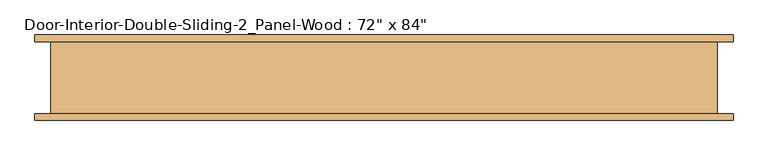
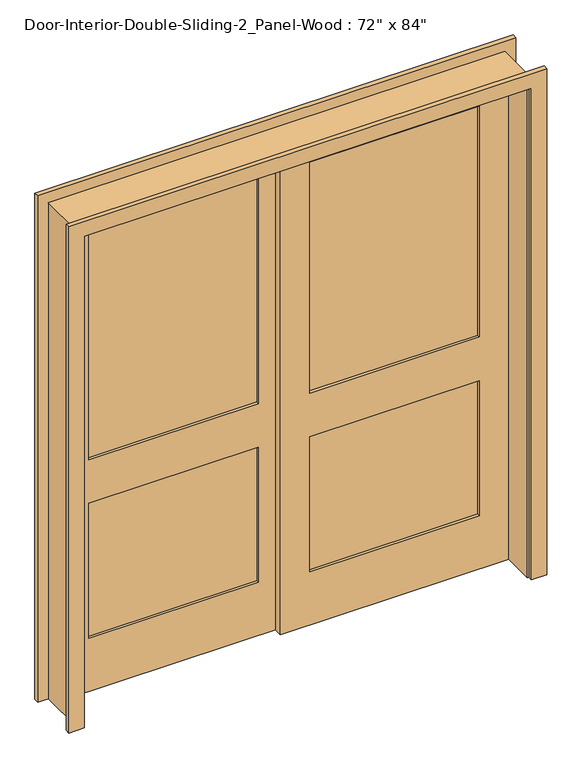
"""IFC4 building model written with IfcOpenShell, lengths in millimetres: door geometry."""

from ifc_helpers import new_model, si_unit, frame, origin, place, context, project, spatial, polyline, outline, extrude, source, transform, mapped, element, save


def door_6868039c(model_context):
    return source(origin(), model_context, "Body", "SweptSolid", [
        extrude(outline(polyline([(793.75, 40.2166667), (95.25, 40.2166667), (95.25, 51.8583333), (793.75, 51.8583333), (793.75, 40.2166667)])), frame((0.0, 0.0, 1009.65), z_axis=(0.0, 0.0, 1.0), x_axis=(1.0, 0.0, 0.0)), (0.0, 0.0, 1.0), 1004.8875),
        extrude(outline(polyline([(793.75, 40.2166667), (95.25, 40.2166667), (95.25, 51.8583333), (793.75, 51.8583333), (793.75, 40.2166667)])), frame((0.0, 0.0, 231.775), z_axis=(0.0, 0.0, 1.0), x_axis=(1.0, 0.0, 0.0)), (0.0, 0.0, 1.0), 587.375),
        extrude(outline(polyline([(2133.6, -25.4), (0.0, -25.4), (0.0, 914.4), (2133.6, 914.4), (2133.6, -25.4)]), holes=[polyline([(2014.5375, 95.25), (2014.5375, 793.75), (1009.65, 793.75), (1009.65, 95.25), (2014.5375, 95.25)]), polyline([(819.15, 95.25), (819.15, 793.75), (231.775, 793.75), (231.775, 95.25), (819.15, 95.25)])]), frame((0.0, 28.575, 0.0), z_axis=(0.0, 1.0, 0.0), x_axis=(0.0, 0.0, 1.0)), (0.0, 0.0, 1.0), 34.925),
        extrude(outline(polyline([(-95.25, 75.1416667), (-793.75, 75.1416667), (-793.75, 86.7833333), (-95.25, 86.7833333), (-95.25, 75.1416667)])), frame((0.0, 0.0, 1009.65), z_axis=(0.0, 0.0, 1.0), x_axis=(1.0, 0.0, 0.0)), (0.0, 0.0, 1.0), 1004.8875),
        extrude(outline(polyline([(-95.25, 75.1416667), (-793.75, 75.1416667), (-793.75, 86.7833333), (-95.25, 86.7833333), (-95.25, 75.1416667)])), frame((0.0, 0.0, 231.775), z_axis=(0.0, 0.0, 1.0), x_axis=(1.0, 0.0, 0.0)), (0.0, 0.0, 1.0), 587.375),
        extrude(outline(polyline([(2133.6, -914.4), (0.0, -914.4), (0.0, 25.4), (2133.6, 25.4), (2133.6, -914.4)]), holes=[polyline([(2014.5375, -793.75), (2014.5375, -95.25), (1009.65, -95.25), (1009.65, -793.75), (2014.5375, -793.75)]), polyline([(819.15, -793.75), (819.15, -95.25), (231.775, -95.25), (231.775, -793.75), (819.15, -793.75)])]), frame((0.0, 63.5, 0.0), z_axis=(0.0, 1.0, 0.0), x_axis=(0.0, 0.0, 1.0)), (0.0, 0.0, 1.0), 34.925),
        extrude(outline(polyline([(0.0, 914.4), (0.0, 939.8), (2159.0, 939.8), (2159.0, -939.8), (0.0, -939.8), (0.0, -914.4), (2133.6, -914.4), (2133.6, 914.4), (0.0, 914.4)])), frame((0.0, -104.775, 0.0), z_axis=(0.0, 1.0, 0.0), x_axis=(0.0, 0.0, 1.0)), (0.0, 0.0, 1.0), 203.2),
        extrude(outline(polyline([(0.0, 920.75), (0.0, 984.25), (2203.45, 984.25), (2203.45, -984.25), (0.0, -984.25), (0.0, -920.75), (2139.95, -920.75), (2139.95, 920.75), (0.0, 920.75)])), frame((0.0, -123.825, 0.0), z_axis=(0.0, 1.0, 0.0), x_axis=(0.0, 0.0, 1.0)), (0.0, 0.0, 1.0), 19.05),
        extrude(outline(polyline([(0.0, 920.75), (0.0, 984.25), (2203.45, 984.25), (2203.45, -984.25), (0.0, -984.25), (0.0, -920.75), (2139.95, -920.75), (2139.95, 920.75), (0.0, 920.75)])), frame((0.0, 98.425, 0.0), z_axis=(0.0, 1.0, 0.0), x_axis=(0.0, 0.0, 1.0)), (0.0, 0.0, 1.0), 19.05),
    ])


if __name__ == "__main__":
    model = new_model("IFC4")
    model_context = context("Model", 3, world=origin())
    ifc_project = project(units=[si_unit("LENGTHUNIT", "METRE", prefix="MILLI")], contexts=[model_context])
    site = spatial("IfcSite", under=ifc_project)
    building = spatial("IfcBuilding", under=site)
    placement = place(None, origin())
    door_shape = door_6868039c(model_context)
    element("IfcDoor", 1, ObjectType="Door-Interior-Double-Sliding-2_Panel-Wood : 72\" x 84\"", at=placement, inside=building, context=model_context, shape_type="MappedRepresentation", body=[
        mapped(door_shape, transform((0.0, 0.0, 0.0), x_axis=(1.0, 0.0, 0.0), y_axis=(0.0, 1.0, 0.0), z_axis=(0.0, 0.0, 1.0))),
    ])
    save(model, "model.ifc")

# Revit data of these elements
# Type "Door-Interior-Double-Sliding-2_Panel-Wood : 72\" x 84\""
#   Type Mark = "8"
#   Assembly Code = "C1020300"
#   Analytic Construction = "Wooden"
#   Top Rail = 0' - 4 11/16"
#   Thickness = 0' - 1 3/8"
#   Thermal Resistance (R) = 2.5876 (h·ft²·°F)/BTU
#   Stiles = 0' - 4 3/4"
#   Rough Width = 6' - 2"
#   Rough Height = 7' - 1"
#   Lock Rail = 0' - 7 1/2"
#   Height = 7' - 0"
#   Width = 6' - 0"
#   Heat Transfer Coefficient (U) = 0.3865 BTU/(h·ft²·°F)
#   Bottom Rail = 0' - 9 1/8"
#   Trim Material = Cherry
#   Panel Material = Cherry
#   Frame Material = Cherry
#   Visual Light Transmittance = 0
#   Solar Heat Gain Coefficient = 0
#   Wall Closure = (empty or 0)
#   Function = (empty or 0)
# Element 1 (IfcDoor, "Door-Interior-Double-Sliding-2_Panel-Wood : 72\" x 84\"")
#   Materials on its faces: "Cherry"
# Materials
#   "Cherry": class "Wood", colour RGB 226 177 128, transparency 0, Description = "Prunus Serotina", Cost = 0
